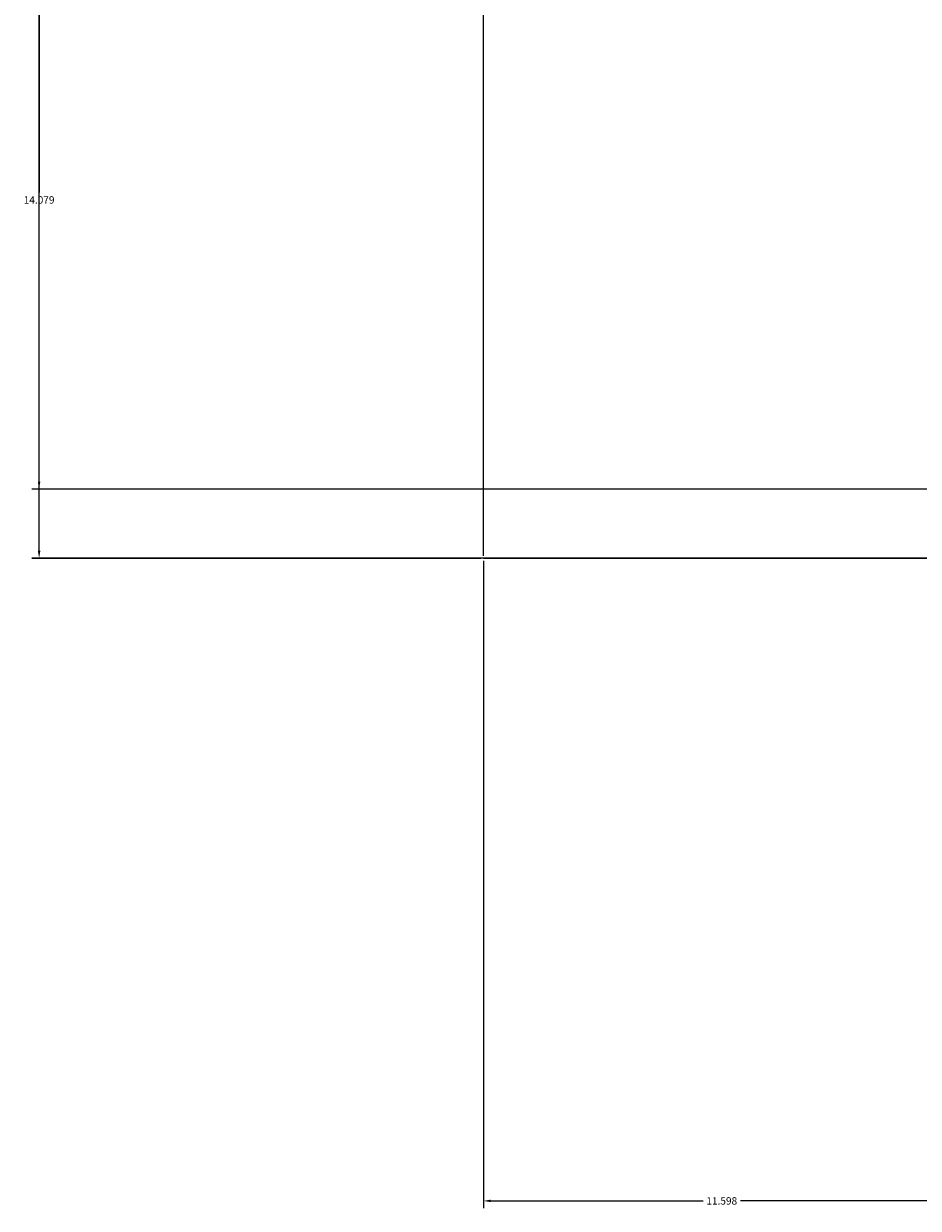
# Model space of a CAD drawing. Units: inches. Extents: x -117 to 121, y -77 to 40.
# Tile 1 of 45: x -117 to -95, y -77 to -48. Entities that reach past the tile are written whole.
import ezdxf

# ---------------------------------------------------------------- set-up
doc = ezdxf.new("R2010")
doc.units = ezdxf.units.IN
doc.header["$MEASUREMENT"] = 0
doc.layers.add('A-ANNO-DIMS', color=2, linetype='Continuous', lineweight=18)
doc.layers.add('A-ELEV', color=7, linetype='Continuous', lineweight=25)
doc.styles.get("Standard").update_dxf_attribs({"font": 'arial.ttf'})
doc.dimstyles.get("Standard").update_dxf_attribs({"dimtxt": 0.18, "dimasz": 0.18, "dimexe": 0.18, "dimexo": 0.0625, "dimgap": 0.09, "dimtad": 0, "dimtih": 1, "dimtoh": 1, "dimdec": 4, "dimzin": 0, "dimdsep": 46, "dimtxsty": 'Standard', "dimcen": 0.09, "dimadec": 0, "dimazin": 0, "dimtfac": 1, "dimtdec": 4, "dimtofl": 0, "dimtmove": 0, "dimatfit": 3, "dimfxl": 1, "dimtolj": 1, "dimtzin": 0, "dimarcsym": 0})

# ---------------------------------------------------------------- blocks, each defined once
blk = doc.blocks.new('*D5')
at = {"layer": 'A-ANNO-DIMS', "color": 0, "lineweight": -2, "transparency": 16777216}
for p, q in [((-94.436, -23.563), (-94.436, -77.193)), ((-106.034, -61.438), (-106.034, -77.193)), ((-105.854, -77.013), (-100.69, -77.013)), ((-94.616, -77.013), (-99.779, -77.013))]:
    blk.add_line(p, q, dxfattribs=at)
at = {"layer": 'A-ANNO-DIMS', "color": 0, "transparency": 16777216}
for points in [[(-105.854, -76.983), (-105.854, -77.043), (-106.034, -77.013)], [(-94.616, -76.983), (-94.616, -77.043), (-94.436, -77.013)]]:
    blk.add_solid(points, dxfattribs=at)
at = {"layer": 'Defpoints', "color": 0, "transparency": 16777216}
for p in [(-94.436, -23.501), (-106.034, -61.376), (-94.436, -77.013)]:
    blk.add_point(p, dxfattribs=at)
at = {"layer": 'A-ANNO-DIMS', "color": 0, "transparency": 16777216, "insert": (-100.235, -77.013), "char_height": 0.18, "attachment_point": 5}
blk.add_mtext('\\A1;11.598', dxfattribs=at)
blk = doc.blocks.new('*D13')
at = {"layer": 'A-ANNO-DIMS', "color": 0, "lineweight": -2, "transparency": 16777216}
for p, q in [((-2.663, 27.063), (-117.024, 27.063)), ((-116.844, 26.883), (-116.844, -16.974)), ((-116.844, -61.196), (-116.844, -17.338)), ((-106.096, -61.376), (-117.024, -61.376))]:
    blk.add_line(p, q, dxfattribs=at)
at = {"layer": 'A-ANNO-DIMS', "color": 0, "transparency": 16777216}
for points in [[(-116.874, 26.883), (-116.814, 26.883), (-116.844, 27.063)], [(-116.874, -61.196), (-116.814, -61.196), (-116.844, -61.376)]]:
    blk.add_solid(points, dxfattribs=at)
at = {"layer": 'Defpoints', "color": 0, "transparency": 16777216}
for p in [(-2.6, 27.063), (-116.844, -61.376), (-106.034, -61.376)]:
    blk.add_point(p, dxfattribs=at)
at = {"layer": 'A-ANNO-DIMS', "color": 0, "transparency": 16777216, "insert": (-116.844, -17.156), "char_height": 0.18, "attachment_point": 5}
blk.add_mtext('\\A1;88.44', dxfattribs=at)
blk = doc.blocks.new('*D18')
at = {"layer": 'A-ANNO-DIMS', "color": 0, "lineweight": -2, "transparency": 16777216}
for p, q in [((-94.498, -23.501), (-117.024, -23.501)), ((-116.844, -23.681), (-116.844, -42.253)), ((-116.844, -61.189), (-116.844, -42.617)), ((-77.826, -61.369), (-117.024, -61.369))]:
    blk.add_line(p, q, dxfattribs=at)
at = {"layer": 'A-ANNO-DIMS', "color": 0, "transparency": 16777216}
for points in [[(-116.874, -23.681), (-116.814, -23.681), (-116.844, -23.501)], [(-116.874, -61.189), (-116.814, -61.189), (-116.844, -61.369)]]:
    blk.add_solid(points, dxfattribs=at)
at = {"layer": 'Defpoints', "color": 0, "transparency": 16777216}
for p in [(-94.436, -23.501), (-116.844, -61.369), (-77.763, -61.369)]:
    blk.add_point(p, dxfattribs=at)
at = {"layer": 'A-ANNO-DIMS', "color": 0, "transparency": 16777216, "insert": (-116.844, -42.435), "char_height": 0.18, "attachment_point": 5}
blk.add_mtext('\\A1;37.87', dxfattribs=at)
blk = doc.blocks.new('*D21')
at = {"layer": 'A-ANNO-DIMS', "color": 0, "lineweight": -2, "transparency": 16777216}
for p, q in [((-106.034, -61.313), (-106.034, 38.61)), ((-105.854, 38.43), (-91.382, 38.43)), ((-75.984, 38.43), (-90.455, 38.43)), ((-75.804, 8.087), (-75.804, 38.61))]:
    blk.add_line(p, q, dxfattribs=at)
at = {"layer": 'A-ANNO-DIMS', "color": 0, "transparency": 16777216}
for points in [[(-105.854, 38.46), (-105.854, 38.4), (-106.034, 38.43)], [(-75.984, 38.46), (-75.984, 38.4), (-75.804, 38.43)]]:
    blk.add_solid(points, dxfattribs=at)
at = {"layer": 'Defpoints', "color": 0, "transparency": 16777216}
for p in [(-75.804, 38.43), (-75.804, 8.025), (-106.034, -61.376)]:
    blk.add_point(p, dxfattribs=at)
at = {"layer": 'A-ANNO-DIMS', "color": 0, "transparency": 16777216, "insert": (-90.919, 38.43), "char_height": 0.18, "attachment_point": 5}
blk.add_mtext('\\A1;30.230', dxfattribs=at)
blk = doc.blocks.new('*D37')
at = {"layer": 'A-ANNO-DIMS', "color": 0, "lineweight": -2, "transparency": 16777216}
for p, q in [((-3.912, -45.613), (-117.024, -45.613)), ((-116.844, -45.793), (-116.844, -52.47)), ((-116.844, -59.512), (-116.844, -52.834)), ((-3.912, -59.692), (-117.024, -59.692))]:
    blk.add_line(p, q, dxfattribs=at)
at = {"layer": 'A-ANNO-DIMS', "color": 0, "transparency": 16777216}
for points in [[(-116.874, -45.793), (-116.814, -45.793), (-116.844, -45.613)], [(-116.874, -59.512), (-116.814, -59.512), (-116.844, -59.692)]]:
    blk.add_solid(points, dxfattribs=at)
at = {"layer": 'Defpoints', "color": 0, "transparency": 16777216}
for p in [(-116.844, -45.613), (-3.85, -45.613), (-3.85, -59.692)]:
    blk.add_point(p, dxfattribs=at)
at = {"layer": 'A-ANNO-DIMS', "color": 0, "transparency": 16777216, "insert": (-116.844, -52.652), "char_height": 0.18, "attachment_point": 5}
blk.add_mtext('\\A1;14.079', dxfattribs=at)

msp = doc.modelspace()

# ---------------------------------------------------------------- linework, layer by layer
at = {"layer": 'A-ELEV'}
msp.add_line((-87.9273, -61.3756), (-106.0338, -61.3756), dxfattribs=at)

# ---------------------------------------------------------------- dimensions: what is measured, and where the dimension line sits
at = {"layer": 'A-ANNO-DIMS'}
for base, p2, picture, middle in [((-75.8037, 38.4297), (-75.8037, 8.0246), '*D21', (-90.9187, 38.4297)), ((-94.4355, -77.0135), (-94.4355, -23.5007), '*D5', (-100.2346, -77.0135))]:
    dim = msp.add_linear_dim(base=base, p1=(-106.0338, -61.3756), p2=p2, dimstyle='Standard', override={"dimdec": 3, "dimlfac": 1, "dimrnd": 0, "dimzin": 0, "dimdsep": 46, "dimlunit": 2}, dxfattribs=at)
    dim.commit()
    dim.dimension.update_dxf_attribs({"geometry": picture, "text_midpoint": middle})
for base, p1, p2, override, picture, middle in [((-116.8438, -61.3756), (-2.6001, 27.0634), (-106.0338, -61.3756), {"dimdec": 2, "dimlfac": 1, "dimrnd": 0, "dimzin": 0, "dimdsep": 46, "dimlunit": 2}, '*D13', (-116.8438, -17.1561)), ((-116.8438, -61.3689), (-94.4355, -23.5007), (-77.7631, -61.3689), {"dimdec": 2, "dimlfac": 1, "dimrnd": 0, "dimzin": 0, "dimdsep": 46, "dimlunit": 2}, '*D18', (-116.8438, -42.4348)), ((-116.843772, -45.612514), (-3.849514, -59.692012), (-3.849514, -45.612514), {"dimdec": 3, "dimlfac": 1, "dimrnd": 0, "dimzin": 0, "dimdsep": 46, "dimlunit": 2}, '*D37', (-116.843772, -52.652263))]:
    dim = msp.add_linear_dim(base=base, p1=p1, p2=p2, angle=90, dimstyle='Standard', override=override, dxfattribs=at)
    dim.commit()
    dim.dimension.update_dxf_attribs({"geometry": picture, "text_midpoint": middle})

doc.saveas('drawing.dxf')
